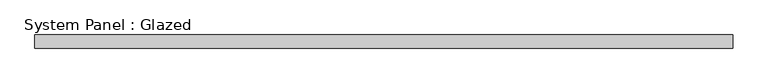
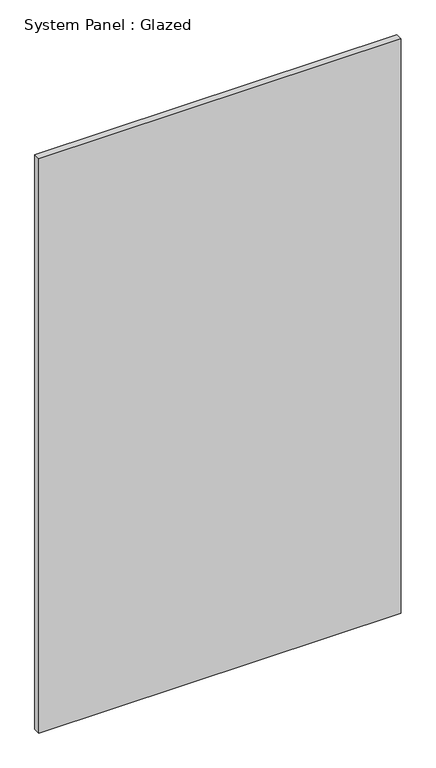
"""IFC4 building model written with IfcOpenShell, lengths in millimetres: plate geometry, System Panel : Glazed."""

from ifc_helpers import new_model, si_unit, origin, origin_with_axes, place, context, project, spatial, polyline, outline, extrude, source, transform, mapped, element, save


def system_panel_glazed_2483beae(model_context):
    return source(origin(), model_context, "Body", "SweptSolid", [
        extrude(outline(polyline([(654.05, 19.05), (-654.05, 19.05), (-654.05, 44.45), (654.05, 44.45), (654.05, 19.05)])), origin_with_axes(), (0.0, 0.0, 1.0), 2190.75),
    ])


if __name__ == "__main__":
    model = new_model("IFC4")
    model_context = context("Model", 3, world=origin())
    ifc_project = project(units=[si_unit("LENGTHUNIT", "METRE", prefix="MILLI")], contexts=[model_context])
    site = spatial("IfcSite", under=ifc_project)
    building = spatial("IfcBuilding", under=site)
    placement = place(None, origin())
    system_panel_glazed_shape = system_panel_glazed_2483beae(model_context)
    element("IfcPlate", 1, ObjectType="System Panel : Glazed", at=placement, inside=building, context=model_context, shape_type="MappedRepresentation", body=[
        mapped(system_panel_glazed_shape, transform((0.0, 0.0, 0.0), x_axis=(1.0, 0.0, 0.0), y_axis=(0.0, 1.0, 0.0), z_axis=(0.0, 0.0, 1.0))),
    ])
    save(model, "model.ifc")

# Revit data of these elements
# Type "System Panel : Glazed"
#   Construction Type Id = "GSP4R"
#   Analytic Construction = "1/8 in Pilkington single glazing"
#   Visual Light Transmittance = 0.9
#   Solar Heat Gain Coefficient = 0.86
#   Heat Transfer Coefficient (U) = 1.18115 BTU/(h·ft²·°F)
#   Define Thermal Properties by = 1
# Element 1 (IfcPlate, "System Panel : Glazed")
#   Materials on its faces: "Glass"
# Materials
#   "Glass": class "Glass", colour RGB 0 128 192, transparency 0.75, Description = "Soda Lime Glass", Cost = 0
